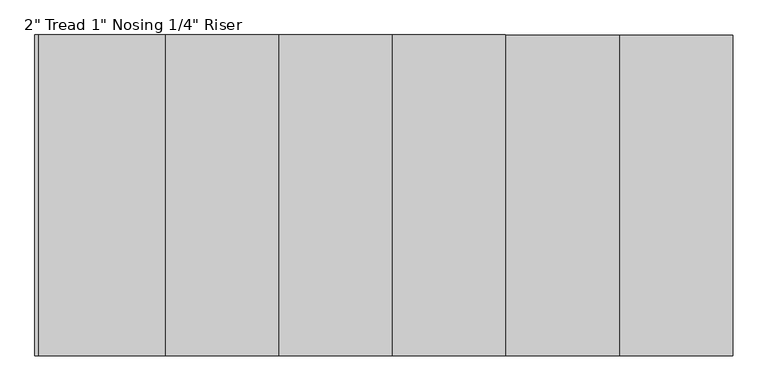
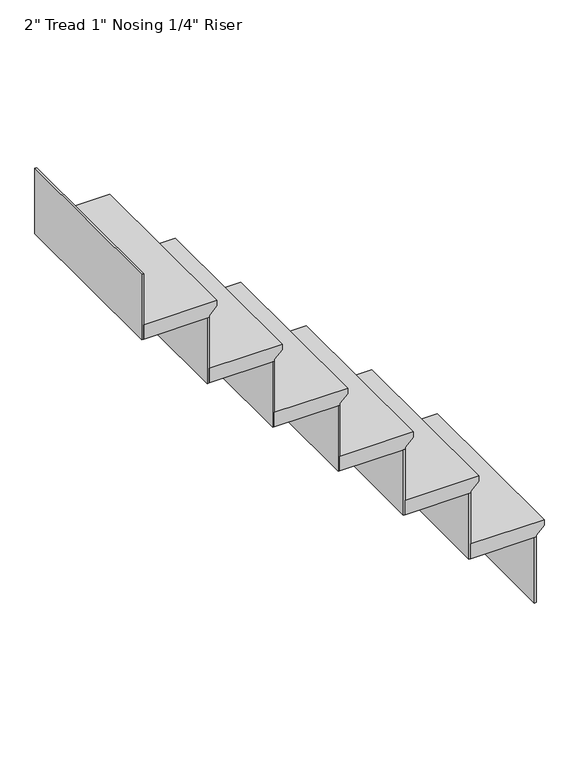
"""IFC4 building model written with IfcOpenShell, lengths in millimetres: stair flight geometry."""

from ifc_helpers import new_model, si_unit, frame, origin, place, context, project, spatial, polyline, outline, extrude, source, transform, mapped, element, save


def stair_flight_0dc73603(model_context):
    return source(origin(), model_context, "Body", "SweptSolid", [
        extrude(outline(polyline([(5029.2, -3732.7409298), (5029.2, -3974.0409298), (4978.4, -3974.0409298), (4978.4, -3758.1409298), (4984.75, -3758.1409298), (5010.15, -3732.7409298), (5029.2, -3732.7409298)])), frame((0.0, -4554.9664375, 0.0), z_axis=(0.0, 1.0, 0.0), x_axis=(0.0, 0.0, 1.0)), (0.0, 0.0, 1.0), 609.6),
        extrude(outline(polyline([(-3764.4909298, -3945.3664375), (-3758.1409298, -3945.3664375), (-3758.1409298, -4554.9664375), (-3764.4909298, -4554.9664375), (-3764.4909298, -3945.3664375)])), frame((0.0, 0.0, 4749.8), z_axis=(0.0, 0.0, 1.0), x_axis=(1.0, 0.0, 0.0)), (0.0, 0.0, 1.0), 228.6),
        extrude(outline(polyline([(-3980.3909298, -3945.3664375), (-3974.0409298, -3945.3664375), (-3974.0409298, -4554.9664375), (-3980.3909298, -4554.9664375), (-3980.3909298, -3945.3664375)])), frame((0.0, 0.0, 4978.4), z_axis=(0.0, 0.0, 1.0), x_axis=(1.0, 0.0, 0.0)), (0.0, 0.0, 1.0), 228.6),
        extrude(outline(polyline([(5257.8, -3948.6409298), (5257.8, -4189.9409298), (5207.0, -4189.9409298), (5207.0, -3974.0409298), (5213.35, -3974.0409298), (5238.75, -3948.6409298), (5257.8, -3948.6409298)])), frame((0.0, -4554.9664375, 0.0), z_axis=(0.0, 1.0, 0.0), x_axis=(0.0, 0.0, 1.0)), (0.0, 0.0, 1.0), 609.6),
        extrude(outline(polyline([(-4196.2909298, -3945.3664375), (-4189.9409298, -3945.3664375), (-4189.9409298, -4554.9664375), (-4196.2909298, -4554.9664375), (-4196.2909298, -3945.3664375)])), frame((0.0, 0.0, 5207.0), z_axis=(0.0, 0.0, 1.0), x_axis=(1.0, 0.0, 0.0)), (0.0, 0.0, 1.0), 228.6),
        extrude(outline(polyline([(5486.4, -4164.5409298), (5486.4, -4405.8409298), (5435.6, -4405.8409298), (5435.6, -4189.9409298), (5441.95, -4189.9409298), (5467.35, -4164.5409298), (5486.4, -4164.5409298)])), frame((0.0, -4554.9664375, 0.0), z_axis=(0.0, 1.0, 0.0), x_axis=(0.0, 0.0, 1.0)), (0.0, 0.0, 1.0), 609.6),
        extrude(outline(polyline([(-4412.1909298, -3945.3664375), (-4405.8409298, -3945.3664375), (-4405.8409298, -4554.9664375), (-4412.1909298, -4554.9664375), (-4412.1909298, -3945.3664375)])), frame((0.0, 0.0, 5435.6), z_axis=(0.0, 0.0, 1.0), x_axis=(1.0, 0.0, 0.0)), (0.0, 0.0, 1.0), 228.6),
        extrude(outline(polyline([(5715.0, -4380.4409298), (5715.0, -4621.7409298), (5664.2, -4621.7409298), (5664.2, -4405.8409298), (5670.55, -4405.8409298), (5695.95, -4380.4409298), (5715.0, -4380.4409298)])), frame((0.0, -4554.9664375, 0.0), z_axis=(0.0, 1.0, 0.0), x_axis=(0.0, 0.0, 1.0)), (0.0, 0.0, 1.0), 609.6),
        extrude(outline(polyline([(-4628.0909298, -3945.3664375), (-4621.7409298, -3945.3664375), (-4621.7409298, -4554.9664375), (-4628.0909298, -4554.9664375), (-4628.0909298, -3945.3664375)])), frame((0.0, 0.0, 5664.2), z_axis=(0.0, 0.0, 1.0), x_axis=(1.0, 0.0, 0.0)), (0.0, 0.0, 1.0), 228.6),
        extrude(outline(polyline([(5943.6, -4596.3409298), (5943.6, -4837.6409298), (5892.8, -4837.6409298), (5892.8, -4621.7409298), (5899.15, -4621.7409298), (5924.55, -4596.3409298), (5943.6, -4596.3409298)])), frame((0.0, -4554.9664375, 0.0), z_axis=(0.0, 1.0, 0.0), x_axis=(0.0, 0.0, 1.0)), (0.0, 0.0, 1.0), 609.6),
        extrude(outline(polyline([(-4843.9909298, -3945.3664375), (-4837.6409298, -3945.3664375), (-4837.6409298, -4554.9664375), (-4843.9909298, -4554.9664375), (-4843.9909298, -3945.3664375)])), frame((0.0, 0.0, 5892.8), z_axis=(0.0, 0.0, 1.0), x_axis=(1.0, 0.0, 0.0)), (0.0, 0.0, 1.0), 228.6),
        extrude(outline(polyline([(-5059.8909298, -3945.3664375), (-5053.5409298, -3945.3664375), (-5053.5409298, -4554.9664375), (-5059.8909298, -4554.9664375), (-5059.8909298, -3945.3664375)])), frame((0.0, 0.0, 6121.4), z_axis=(0.0, 0.0, 1.0), x_axis=(1.0, 0.0, 0.0)), (0.0, 0.0, 1.0), 228.6),
        extrude(outline(polyline([(6172.2, -4812.2409298), (6172.2, -5053.5409298), (6121.4, -5053.5409298), (6121.4, -4837.6409298), (6127.75, -4837.6409298), (6153.15, -4812.2409298), (6172.2, -4812.2409298)])), frame((0.0, -4554.9664375, 0.0), z_axis=(0.0, 1.0, 0.0), x_axis=(0.0, 0.0, 1.0)), (0.0, 0.0, 1.0), 609.6),
    ])


if __name__ == "__main__":
    model = new_model("IFC4")
    model_context = context("Model", 3, world=origin())
    ifc_project = project(units=[si_unit("LENGTHUNIT", "METRE", prefix="MILLI")], contexts=[model_context])
    site = spatial("IfcSite", under=ifc_project)
    building = spatial("IfcBuilding", under=site)
    placement = place(None, origin())
    stair_flight_shape = stair_flight_0dc73603(model_context)
    element("IfcStairFlight", 1, ObjectType="2\" Tread 1\" Nosing 1/4\" Riser", at=placement, inside=building, context=model_context, shape_type="MappedRepresentation", body=[
        mapped(stair_flight_shape, transform((0.0, 0.0, 0.0), x_axis=(1.0, 0.0, 0.0), y_axis=(0.0, 1.0, 0.0), z_axis=(0.0, 0.0, 1.0))),
    ])
    save(model, "model.ifc")
